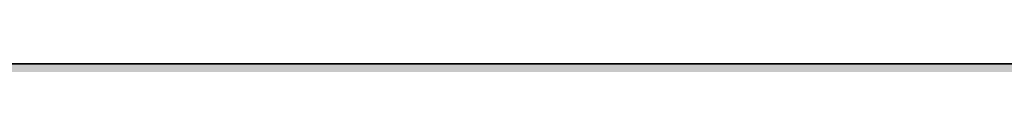
# Model space of a CAD drawing. Units: inches. Extents: x 2091 to 2899, y 967 to 2217.
# Tile 73 of 256: x 2214.757 to 2217.572, y 1099.919 to 1099.919. Entities that reach past the tile are written whole.
import ezdxf

# ---------------------------------------------------------------- set-up
doc = ezdxf.new("R2010")
doc.units = ezdxf.units.IN
doc.layers.add('A-WALL-PATT', color=141, linetype='Continuous', lineweight=13, true_color=0xadddf7)
doc.layers.add('L-SITE-WALL', color=7, linetype='Continuous', lineweight=35)

msp = doc.modelspace()

# ---------------------------------------------------------------- hatches: boundary and pattern name
at = {"layer": 'A-WALL-PATT'}
h = msp.add_hatch(color=256, dxfattribs=at)
h.dxf.hatch_style = 1
h.paths.add_polyline_path([(2212.1436, 1941.4191), (2387.6436, 1941.4191), (2387.6436, 1824.4191), (2392.1436, 1824.4191), (2392.1436, 1941.4191), (2609.6436, 1941.4191), (2609.6436, 1825.9191), (2614.1436, 1825.9191), (2614.1436, 1941.4191), (2794.1436, 1941.4191), (2794.1436, 1928.7622), (2803.1436, 1928.7622), (2803.1436, 2050.9191), (2203.1436, 2050.9191), (2203.1436, 1900.7579), (2212.1436, 1900.7579)])
h.paths.add_polyline_path([(2212.1436, 1945.9191), (2212.1436, 2041.9191), (2794.1436, 2041.9191), (2794.1436, 1945.9191), (2402.2482, 1945.9191), (2401.1024, 1945.7758), (2398.7024, 1945.7758)], flags=16)
h.paths.add_polyline_path([(2230.2299, 1948.0628), (2227.3499, 1949.5028), (2225.9099, 1951.9028), (2223.9899, 1952.8628), (2223.0299, 1955.2628), (2222.0699, 1959.5828), (2222.0699, 1963.4228), (2223.0299, 1965.6628), (2223.9899, 1965.3428), (2225.5859, 1963.8607), (2226.9115, 1964.9573), (2226.9489, 1965.9388), (2227.7783, 1966.9521), (2228.1999, 1968.8787), (2230.7099, 1964.8628), (2233.5899, 1966.3028), (2233.6073, 1966.3319), (2233.7727, 1964.9382), (2234.6338, 1963.6765), (2235.0299, 1963.9028), (2236.282, 1965.5724), (2235.9899, 1962.9428), (2237.9545, 1957.54), (2238.3899, 1957.9028), (2239.2159, 1960.3058), (2238.6546, 1966.385), (2238.6928, 1966.4381), (2238.8406, 1967.4997), (2238.7803, 1967.6875), (2238.8805, 1967.7868), (2238.6669, 1966.2518), (2239.2159, 1960.3058), (2238.3899, 1957.9028), (2236.9499, 1956.7028), (2234.5499, 1949.9828)], flags=0)
h.paths.add_polyline_path([(2278.012, 1948.0628), (2276.4964, 1947.8733), (2275.8498, 1947.6886), (2274.652, 1947.1028)], flags=0)
h.paths.add_polyline_path([(2269.852, 1955.7428), (2268.2762, 1956.6293), (2270.8673, 1956.3484), (2269.372, 1958.1428), (2268.715, 1959.1923), (2270.5698, 1958.7286), (2268.5807, 1961.9061), (2270.812, 1960.8919), (2270.812, 1963.4228), (2271.3933, 1964.7793), (2270.2918, 1966.1562), (2271.772, 1965.6628), (2272.1414, 1966.5248), (2273.9298, 1965.9286), (2275.6304, 1968.0543), (2276.3319, 1966.7219), (2276.5204, 1966.9521), (2276.942, 1968.8787), (2277.7343, 1967.6111), (2278.1399, 1969.4645), (2279.6591, 1967.0337), (2280.412, 1966.7828), (2280.9493, 1967.5888), (2281.6098, 1967.3686), (2282.1333, 1968.1538), (2282.3492, 1966.3334), (2282.3498, 1966.3326), (2283.4076, 1968.0954), (2283.7126, 1965.524), (2284.3202, 1964.6338), (2284.5118, 1964.8892), (2284.235, 1965.7048), (2284.5005, 1967.319), (2284.9079, 1965.4174), (2285.3963, 1966.0686), (2285.4328, 1966.2906), (2285.4733, 1966.1713), (2286.3539, 1967.3454), (2286.222, 1966.1582), (2287.6635, 1968.0802), (2287.714, 1968.4428), (2288.4816, 1969.0167), (2288.574, 1968.7289), (2288.9175, 1969.069), (2288.6068, 1966.8376), (2288.9287, 1963.3513), (2288.935, 1963.3568), (2288.9297, 1963.3404), (2289.0153, 1962.4139), (2290.1112, 1963.8751), (2290.1328, 1963.9426), (2290.2177, 1964.0171), (2290.1112, 1963.8751), (2289.1558, 1960.8916), (2288.594, 1959.2572), (2288.572, 1959.1028), (2289.532, 1960.5428), (2290.012, 1962.4628), (2290.1918, 1962.6427), (2289.7698, 1959.6886), (2286.8898, 1957.2886), (2284.4898, 1950.5686), (2283.3147, 1950.0463), (2283.292, 1949.9828), (2280.2901, 1948.6486), (2281.1298, 1948.6486), (2282.5698, 1948.1686), (2283.2047, 1948.0628), (2278.972, 1948.0628), (2276.092, 1949.5028), (2274.652, 1951.9028), (2272.732, 1952.8628)], flags=0)
h.paths.add_polyline_path([(2271.1589, 1958.0218), (2272.9698, 1955.8486), (2272.0098, 1960.1686), (2272.0098, 1964.0086), (2272.6244, 1965.4427), (2274.328, 1963.8607), (2275.6536, 1964.9573), (2275.6377, 1964.5391), (2277.4122, 1966.0069), (2277.033, 1965.1568), (2276.8299, 1964.9756), (2276.766, 1963.295), (2277.4496, 1962.6602), (2279.452, 1964.8628), (2282.332, 1966.3028), (2283.5298, 1966.8886), (2283.2945, 1966.7709), (2283.913, 1963.8847), (2284.8992, 1964.4483), (2284.732, 1962.9428), (2286.6966, 1957.54), (2287.132, 1957.9028), (2287.5419, 1959.0954), (2287.7794, 1958.4423), (2285.6827, 1956.6951), (2285.8765, 1959.7953), (2284.732, 1962.9428), (2284.8992, 1964.4483), (2283.913, 1963.8847), (2284.2238, 1962.4341), (2283.4244, 1963.6055), (2281.6098, 1962.5686), (2281.1298, 1960.1686), (2282.0898, 1956.3286), (2283.0498, 1952.9686), (2282.5698, 1950.5686), (2280.1698, 1948.6486), (2279.8833, 1948.7919), (2278.972, 1948.0628), (2278.972, 1949.0228), (2278.6723, 1949.3974), (2277.2898, 1950.0886), (2275.8498, 1952.4886), (2273.9298, 1953.4486), (2272.4898, 1954.8886), (2271.9216, 1954.8886), (2271.772, 1955.2628)], flags=0)
h.paths.add_polyline_path([(2311.9941, 1955.7428), (2312.0627, 1955.6742), (2312.0551, 1955.7085)], flags=0)
h.paths.add_polyline_path([(2331.9561, 1963.9518), (2333.3961, 1965.3918), (2331.0771, 1963.3568), (2330.9986, 1963.1115)], flags=0)
h.paths.add_polyline_path([(2310.5541, 1954.3028), (2307.0398, 1956.2799), (2310.7629, 1955.8763), (2312.4741, 1953.8228), (2313.4341, 1951.4228), (2315.3541, 1950.4628), (2316.7941, 1948.0628), (2317.4661, 1947.7268), (2319.3687, 1947.9646), (2317.7541, 1949.9828), (2317.5695, 1950.6105), (2316.7941, 1951.9028), (2314.8741, 1952.8628), (2313.9141, 1955.2628), (2311.5141, 1958.1428), (2309.3755, 1961.5592), (2311.5141, 1960.3371), (2311.5141, 1961.9828), (2310.6047, 1963.1196), (2311.7266, 1962.4785), (2312.4183, 1964.0926), (2312.256, 1964.2955), (2313.1941, 1963.9828), (2313.9141, 1965.6628), (2314.6468, 1965.4186), (2315.3541, 1966.3028), (2316.7941, 1967.7428), (2316.1574, 1966.9469), (2317.0341, 1965.2819), (2317.2226, 1965.5121), (2317.777, 1968.0458), (2318.4741, 1966.7219), (2318.6626, 1966.9521), (2319.0842, 1968.8787), (2321.207, 1965.4821), (2322.1614, 1966.9137), (2322.5541, 1966.7828), (2322.786, 1967.1306), (2322.8816, 1966.3243), (2323.312, 1965.7217), (2323.6513, 1965.8914), (2324.3965, 1967.1334), (2324.6569, 1964.9382), (2324.972, 1964.4766), (2325.3873, 1967.0015), (2325.9408, 1964.4183), (2327.2289, 1966.1358), (2327.1663, 1965.5724), (2328.0591, 1966.7628), (2328.2246, 1966.2475), (2329.668, 1967.6769), (2329.6646, 1967.6875), (2329.7648, 1967.7868), (2329.5511, 1966.2518), (2330.1001, 1960.3058), (2329.3328, 1958.0735), (2329.3131, 1957.9352), (2329.6341, 1958.2028), (2330.2341, 1959.1028), (2330.7141, 1961.0228), (2331.0341, 1961.3428), (2330.7141, 1959.1028), (2329.6341, 1958.2028), (2329.2741, 1957.6628), (2327.7121, 1956.3611), (2325.4341, 1949.9828), (2324.3338, 1949.4937), (2323.9941, 1948.5428), (2319.6741, 1946.6228), (2316.7941, 1948.0628), (2315.3541, 1950.4628), (2313.4341, 1951.4228)], flags=0)
h.paths.add_polyline_path([(2321.3357, 1947.952), (2321.1141, 1948.0628), (2321.1141, 1949.0228), (2319.1941, 1951.4228), (2316.7941, 1959.5828), (2316.6632, 1959.5828), (2315.3541, 1958.1428), (2314.3941, 1958.1428), (2313.1483, 1958.7091), (2312.9541, 1959.5828), (2312.9541, 1960.8919), (2315.8341, 1959.5828), (2316.6632, 1959.5828), (2317.3147, 1960.2994), (2315.0302, 1962.4207), (2316.3558, 1963.5173), (2316.3723, 1963.9516), (2316.4702, 1963.8607), (2317.7958, 1964.9573), (2317.7552, 1963.8897), (2319.1751, 1965.1568), (2319.4984, 1965.8814), (2321.1141, 1965.3428), (2323.2359, 1962.3724), (2325.6863, 1963.7726), (2325.5428, 1962.4806), (2325.1988, 1963.494), (2324.4785, 1963.0824), (2324.926, 1960.9941), (2324.0781, 1962.2365), (2322.4148, 1961.286), (2322.0741, 1959.5828), (2323.0341, 1955.7428), (2323.9941, 1952.3828), (2323.5141, 1949.9828), (2322.1427, 1948.8856), (2322.0741, 1948.5428)], flags=0)
h.paths.add_polyline_path([(2320.2075, 1963.3375), (2320.1541, 1963.4228), (2320.3941, 1963.5428)], flags=0)
h.paths.add_polyline_path([(2353.8505, 1965.8105), (2354.0305, 1965.7505), (2354.3305, 1966.4505), (2354.3305, 1966.9305)], flags=0)
h.paths.add_polyline_path([(2359.0206, 1969.0264), (2359.0984, 1968.9019), (2359.2335, 1969.5195), (2359.2335, 1969.9995)], flags=0)
h.paths.add_polyline_path([(2358.2567, 1966.6817), (2357.9836, 1966.348), (2358.2113, 1966.1462), (2358.4105, 1966.3896)], flags=0)
h.paths.add_polyline_path([(2357.7685, 1966.0588), (2357.7322, 1965.105), (2357.751, 1965.1206), (2357.7695, 1965.6065), (2357.7695, 1966.0578)], flags=0)
h.paths.add_polyline_path([(2359.1115, 1965.3045), (2359.1115, 1964.8245), (2359.8445, 1966.4675), (2359.8445, 1966.9475)], flags=0)
h.paths.add_polyline_path([(2360.2237, 1966.6214), (2360.6985, 1969.3625), (2360.6985, 1969.8425), (2360.2105, 1967.0255), (2360.2105, 1966.6425)], flags=0)
h.paths.add_polyline_path([(2363.4505, 1967.8905), (2363.4505, 1968.3705), (2362.4905, 1966.9305), (2362.656, 1966.6988)], flags=0)
h.paths.add_polyline_path([(2364.4755, 1966.0788), (2365.8505, 1968.3705), (2365.8505, 1968.8505), (2364.428, 1966.4796)], flags=0)
h.paths.add_polyline_path([(2366.3135, 1965.8525), (2366.3667, 1965.6958), (2366.8025, 1968.3455), (2366.8025, 1968.8255)], flags=0)
h.paths.add_polyline_path([(2367.1653, 1965.8035), (2367.2905, 1966.9305), (2367.2905, 1967.4105), (2367.1027, 1965.7201)], flags=0)
h.paths.add_polyline_path([(2370.0365, 1959.9735), (2371.0135, 1963.0245), (2371.0135, 1963.5045), (2370.0365, 1960.4535)], flags=0)
h.paths.add_polyline_path([(2371.6105, 1960.2105), (2372.5705, 1961.6505), (2372.5705, 1962.1305), (2371.8025, 1960.9785)], flags=0)
h.paths.add_polyline_path([(2350.8737, 1956.0051), (2351.9305, 1955.8905), (2354.4905, 1953.3305), (2353.8505, 1954.9305), (2351.4505, 1957.8105), (2347.9355, 1963.4255), (2347.9355, 1963.9055), (2351.4505, 1958.2905), (2353.7051, 1955.585), (2352.8905, 1959.2505), (2352.8905, 1959.7305), (2352.8905, 1961.9248), (2356.7305, 1959.7305), (2358.4545, 1961.6268), (2354.8105, 1965.0105), (2355.0309, 1965.2859), (2358.6911, 1961.8871), (2361.5305, 1965.0105), (2364.3765, 1966.4335), (2364.5244, 1965.1869), (2365.4545, 1963.8242), (2365.8811, 1964.068), (2365.3705, 1966.4505), (2365.3705, 1966.9305), (2366.8105, 1960.2105), (2366.8105, 1959.7305), (2366.3887, 1952.9814), (2367.7705, 1956.8505), (2368.6412, 1957.5761), (2366.8105, 1962.6105), (2366.8105, 1963.0905), (2368.7752, 1957.6877), (2369.2105, 1958.0505), (2370.0016, 1960.3519), (2369.4752, 1966.0527), (2369.5135, 1966.1058), (2369.5142, 1966.1109), (2369.4752, 1966.5327), (2369.5135, 1966.5858), (2369.6146, 1967.3126), (2369.1825, 1968.6585), (2369.1825, 1969.1385), (2369.601, 1967.8352), (2369.7012, 1967.9345), (2369.7179, 1968.0547), (2370.1452, 1968.3741), (2369.7787, 1968.0112), (2369.7012, 1967.4545), (2370.4682, 1968.214), (2369.6749, 1967.2658), (2369.5142, 1966.1109), (2370.0365, 1960.4535), (2370.0365, 1959.9735), (2369.4418, 1958.2432), (2370.6505, 1959.2505), (2371.0458, 1962.0176), (2371.1305, 1962.1305), (2370.6505, 1958.7705), (2367.7705, 1956.3705), (2365.3705, 1949.6505), (2362.0791, 1948.1876), (2363.4505, 1947.7305), (2361.0505, 1947.7305), (2360.0905, 1947.7305), (2357.1039, 1947.3572), (2360.0905, 1948.2105), (2358.1705, 1949.1705), (2356.7305, 1951.5705), (2354.8105, 1952.5305), (2351.9305, 1955.4105)], flags=0)
h.paths.add_polyline_path([(2361.0505, 1948.6905), (2359.1305, 1951.0905), (2356.7305, 1959.2505), (2355.7705, 1959.2505), (2352.8905, 1960.5596), (2352.8905, 1961.4448), (2355.8905, 1959.7305), (2356.7305, 1959.7305), (2356.8372, 1959.3678), (2361.5305, 1964.5305), (2363.2484, 1965.3894), (2364.9253, 1963.0418), (2362.4905, 1961.6505), (2362.0639, 1959.5172), (2362.9705, 1955.8905), (2363.9305, 1952.5305), (2363.9305, 1952.0505), (2363.4505, 1949.6505), (2361.0505, 1947.7305)], flags=0)
h.paths.add_polyline_path([(2359.1305, 1951.5705), (2359.2905, 1951.3705), (2361.0505, 1954.4505), (2361.0505, 1954.9305)], flags=0)
h.paths.add_polyline_path([(2357.2195, 1966.5455), (2356.7925, 1968.8145), (2356.7925, 1969.2945), (2357.2195, 1967.0255)], flags=0)
h.paths.add_polyline_path([(2361.0505, 1954.4505), (2361.5305, 1958.7705), (2361.5305, 1959.2505), (2361.0505, 1954.9305)], flags=0)
h.paths.add_polyline_path([(2402.5483, 1948.4861), (2402.3024, 1948.4158), (2402.5904, 1948.4158)], flags=0)
h.paths.add_polyline_path([(2394.1424, 1956.0958), (2395.6851, 1954.5532), (2396.7205, 1953.9707), (2396.0624, 1955.6158), (2395.2414, 1956.6011), (2395.8789, 1956.4417), (2395.1024, 1959.9358), (2395.1024, 1963.7758), (2396.0624, 1966.0158), (2397.0224, 1965.6958), (2398.6185, 1964.2138), (2399.9441, 1965.3103), (2399.9814, 1966.2918), (2400.8109, 1967.3052), (2401.2325, 1969.2317), (2403.5379, 1965.543), (2403.942, 1967.3893), (2404.7024, 1967.1358), (2405.4603, 1966.0748), (2406.6224, 1966.6558), (2406.6399, 1966.6849), (2406.8052, 1965.2912), (2406.9257, 1965.1147), (2407.3424, 1964.9758), (2407.8743, 1965.7737), (2408.1691, 1964.3981), (2409.3146, 1965.9254), (2409.2175, 1965.0511), (2409.4452, 1963.1312), (2410.3064, 1961.8695), (2410.7024, 1962.0958), (2411.4423, 1963.0823), (2411.1654, 1963.8978), (2411.6164, 1966.6398), (2411.7254, 1966.7911), (2411.8732, 1967.8527), (2411.8129, 1968.0405), (2411.9131, 1968.1398), (2411.6994, 1966.6048), (2412.2484, 1960.6588), (2413.2254, 1963.7098), (2414.3779, 1964.7212), (2414.5132, 1965.6927), (2414.4529, 1965.8805), (2414.5531, 1965.9798), (2414.3779, 1964.7212), (2414.5198, 1964.8457), (2414.3654, 1964.6311), (2414.3394, 1964.4448), (2414.8884, 1958.4988), (2414.0624, 1956.0958), (2412.6224, 1954.8958), (2410.1714, 1948.0329), (2410.0167, 1948.0844), (2405.9024, 1946.2558), (2405.9024, 1947.2158), (2405.2043, 1948.0886), (2404.2224, 1948.4158), (2403.2624, 1948.4158), (2400.3824, 1949.8558), (2399.6624, 1951.0558), (2397.9824, 1952.7358), (2397.0224, 1953.2158), (2395.6851, 1954.5532), (2392.6568, 1956.2569)], flags=0)
h.paths.add_polyline_path([(2409.0857, 1964.4074), (2409.1304, 1964.2757), (2409.2624, 1964.4958)], flags=0)
h.paths.add_polyline_path([(2397.7424, 1961.6158), (2398.7024, 1963.8558), (2399.6624, 1963.5358), (2401.4266, 1965.741), (2401.7914, 1966.5588), (2402.0714, 1965.0708), (2402.8355, 1964.3934), (2403.2624, 1964.9149), (2403.3381, 1964.7711), (2402.6155, 1963.9762), (2402.4986, 1960.9022), (2403.543, 1959.9325), (2404.4132, 1960.8897), (2404.7024, 1962.3358), (2407.9163, 1964.1724), (2409.5202, 1961.9269), (2410.9871, 1957.893), (2411.4224, 1958.2558), (2412.048, 1960.0756), (2412.4103, 1959.0791), (2411.6756, 1958.4668), (2411.6624, 1958.2558), (2411.6261, 1958.4255), (2409.9824, 1957.0558), (2407.5824, 1950.3358), (2403.2624, 1948.4158), (2403.2624, 1949.3758), (2401.3424, 1951.7758), (2399.4165, 1958.324), (2397.7424, 1959.0849), (2397.7424, 1959.9701), (2397.1024, 1960.3358), (2397.7424, 1960.0449)], flags=0)
h.paths.add_polyline_path([(2405.9024, 1952.9758), (2405.9504, 1953.4078), (2406.0167, 1953.1758)], flags=0)
h.paths.add_polyline_path([(2449.8178, 1967.114), (2449.7523, 1967.1358), (2449.7937, 1967.0779)], flags=0)
h.paths.add_polyline_path([(2451.6977, 1966.6181), (2451.7409, 1966.6901), (2451.6921, 1966.6657)], flags=0)
h.paths.add_polyline_path([(2454.3436, 1965.7376), (2455.7523, 1967.6158), (2455.9923, 1968.0958), (2454.3645, 1965.9254)], flags=0)
h.paths.add_polyline_path([(2457.5473, 1968.8638), (2457.7873, 1969.3438), (2457.0543, 1968.7958), (2457.0076, 1968.4603)], flags=0)
h.paths.add_polyline_path([(2456.9218, 1967.8567), (2456.8022, 1968.229), (2456.723, 1967.6598)], flags=0)
h.paths.add_polyline_path([(2457.3023, 1967.3768), (2457.5423, 1967.8568), (2456.8103, 1966.8398), (2456.7405, 1966.7002), (2456.749, 1966.6081)], flags=0)
h.paths.add_polyline_path([(2458.2753, 1963.7098), (2458.1553, 1963.3352), (2460.3543, 1965.2648), (2460.5943, 1965.7448)], flags=0)
h.paths.add_polyline_path([(2458.3923, 1962.8158), (2458.3641, 1962.6182), (2459.5923, 1964.2558), (2459.8323, 1964.7358)], flags=0)
h.paths.add_polyline_path([(2459.3523, 1962.8158), (2459.2723, 1962.4958), (2460.0723, 1963.2958), (2460.3123, 1963.7758)], flags=0)
h.paths.add_polyline_path([(2458.6803, 1960.6078), (2458.6323, 1960.4158), (2459.5923, 1961.8558), (2459.8323, 1962.3358)], flags=0)
h.paths.add_polyline_path([(2437.8382, 1956.2427), (2439.1923, 1956.0958), (2441.3523, 1953.9358), (2440.8723, 1955.1358), (2438.4723, 1958.0158), (2438.0716, 1958.656), (2438.7123, 1958.4958), (2440.6396, 1956.1831), (2439.9123, 1959.4558), (2439.9123, 1963.2958), (2441.3523, 1966.6558), (2441.5923, 1967.1358), (2441.1123, 1966.0158), (2442.0723, 1965.6958), (2443.989, 1968.0917), (2444.2413, 1966.7508), (2444.9168, 1966.1519), (2445.6766, 1967.0801), (2446.2553, 1969.7248), (2446.4953, 1970.2048), (2446.2824, 1969.2317), (2447.3627, 1967.5033), (2447.7203, 1969.5678), (2447.9603, 1970.0478), (2447.4855, 1967.3068), (2448.7923, 1965.2158), (2448.4723, 1964.8638), (2448.5523, 1964.7358), (2451.4521, 1966.1857), (2451.6151, 1964.8112), (2452.3079, 1963.7962), (2453.2345, 1964.3257), (2454.0723, 1960.4158), (2453.6287, 1953.3177), (2454.7923, 1956.5758), (2455.0323, 1957.0558), (2455.7188, 1957.6279), (2453.8323, 1962.8158), (2453.941, 1963.7936), (2453.3353, 1965.5778), (2453.8243, 1968.5508), (2454.0643, 1969.0308), (2453.5753, 1966.0578), (2454.0403, 1964.6879), (2453.8323, 1962.8158), (2455.7188, 1957.6279), (2456.3672, 1958.1682), (2457.0583, 1960.1788), (2457.2983, 1960.6588), (2456.4723, 1958.2558), (2457.7177, 1959.2937), (2457.6723, 1958.9758), (2454.89, 1956.6572), (2453.6141, 1953.0849), (2453.5923, 1952.7358), (2453.3523, 1952.2558), (2453.3596, 1952.3722), (2452.6323, 1950.3358), (2452.3923, 1949.8558), (2449.2038, 1948.4387), (2450.7123, 1947.9358), (2448.0723, 1947.9358), (2447.1123, 1947.9358), (2444.5523, 1947.6158), (2447.1996, 1948.3722), (2445.1923, 1949.3758), (2443.7523, 1951.7758), (2441.8323, 1952.7358), (2438.9523, 1955.6158)], flags=0)
h.paths.add_polyline_path([(2443.9923, 1959.9358), (2444.0403, 1959.7726), (2444.1216, 1959.862)], flags=0)
h.paths.add_polyline_path([(2442.9123, 1959.9358), (2443.0323, 1959.9358), (2442.4457, 1960.2025)], flags=0)
h.paths.add_polyline_path([(2444.9829, 1965.0197), (2445.2793, 1965.2648), (2445.5193, 1965.7448), (2444.994, 1965.3103)], flags=0)
h.paths.add_polyline_path([(2446.1333, 1965.0298), (2446.3304, 1965.4715), (2444.9703, 1964.2578), (2444.7303, 1963.7778)], flags=0)
h.paths.add_polyline_path([(2442.7923, 1959.4558), (2443.7523, 1959.4558), (2446.1523, 1951.2958), (2446.4123, 1951.7508), (2446.3923, 1951.7758), (2448.0806, 1954.7303), (2448.5523, 1958.9758), (2441.8323, 1965.2158), (2442.1549, 1965.6191), (2448.7923, 1959.4558), (2448.3123, 1955.1358), (2448.0723, 1954.6558), (2446.4123, 1951.7508), (2448.3123, 1949.3758), (2448.3123, 1948.4158), (2450.5409, 1950.1987), (2450.9523, 1952.2558), (2449.9923, 1955.6158), (2449.0323, 1959.4558), (2449.5123, 1961.8558), (2449.7523, 1962.3358), (2449.6749, 1961.9487), (2452.9945, 1963.8457), (2453.0644, 1963.5194), (2452.8846, 1963.7829), (2449.6749, 1961.9487), (2449.2723, 1959.9358), (2450.2323, 1956.0958), (2451.1923, 1952.7358), (2450.7123, 1950.3358), (2450.4723, 1949.8558), (2448.0723, 1947.9358), (2448.0723, 1948.5358), (2445.4323, 1949.8558), (2443.9923, 1952.2558), (2442.0723, 1953.2158), (2441.1123, 1955.6158), (2440.1523, 1959.9358), (2440.1523, 1960.6558)], flags=0)
h.paths.add_polyline_path([(2456.6923, 1966.9858), (2457.6083, 1968.0808), (2457.8483, 1968.5608), (2456.9323, 1967.4658)], flags=0)
h.paths.add_polyline_path([(2489.8966, 1966.5802), (2489.9429, 1966.1893), (2490.7475, 1967.5302), (2491.3191, 1968.9512)], flags=0)
h.paths.add_polyline_path([(2473.5625, 1956.4071), (2477.14, 1956.0193), (2476.9553, 1956.2408), (2475.108, 1957.2801), (2476.3475, 1956.9702), (2475.1869, 1958.8242), (2476.9191, 1958.3912), (2475.4116, 1960.7993), (2477.7875, 1959.7193), (2477.7875, 1962.2502), (2477.6374, 1962.4379), (2477.8226, 1962.3321), (2478.3591, 1963.5841), (2478.3591, 1963.6712), (2477.3243, 1964.9646), (2478.7148, 1964.5011), (2479.3191, 1965.9112), (2480.2791, 1965.5912), (2481.784, 1967.4722), (2482.1165, 1965.7052), (2482.8806, 1965.0278), (2483.2093, 1965.4294), (2483.2202, 1965.7151), (2483.0759, 1965.989), (2483.7118, 1966.7658), (2484.1305, 1968.6792), (2484.7021, 1970.1002), (2484.4892, 1969.1271), (2486.5029, 1965.9051), (2487.3875, 1965.6102), (2488.1534, 1966.7591), (2488.717, 1965.9701), (2489.2001, 1966.2116), (2489.3307, 1965.111), (2490.3939, 1963.6225), (2490.6608, 1963.775), (2490.4939, 1964.5536), (2490.9231, 1963.9248), (2491.3191, 1964.1512), (2491.3334, 1964.1702), (2491.2105, 1964.5322), (2491.2818, 1964.9655), (2491.4258, 1964.2934), (2494.0765, 1967.8276), (2494.4979, 1966.5149), (2494.5982, 1966.6142), (2494.6895, 1967.2702), (2495.1067, 1967.5822), (2495.1298, 1967.7481), (2495.0696, 1967.9359), (2495.1698, 1968.0351), (2495.0318, 1967.0436), (2495.7538, 1967.7587), (2494.9821, 1966.6864), (2494.9561, 1966.5002), (2495.479, 1960.8369), (2495.9105, 1962.1842), (2496.4821, 1963.6052), (2496.0727, 1962.3266), (2496.7689, 1962.9375), (2496.5991, 1962.7112), (2496.1191, 1959.3512), (2496.7329, 1960.2718), (2496.9875, 1961.2902), (2497.5591, 1962.7112), (2497.0791, 1960.7912), (2496.5075, 1959.3702), (2495.5475, 1957.9302), (2492.7588, 1955.6064), (2490.8391, 1950.2312), (2490.2675, 1948.8102), (2485.9475, 1946.8902), (2483.0675, 1948.3302), (2481.6275, 1950.7302), (2479.7075, 1951.6902), (2476.8275, 1954.5702)], flags=0)
h.paths.add_polyline_path([(2485.577, 1948.3134), (2485.5591, 1948.3112), (2485.5788, 1948.3112)], flags=0)
h.paths.add_polyline_path([(2478.6451, 1954.5512), (2478.109, 1956.9633), (2479.3191, 1955.5112), (2480.2791, 1953.1112), (2482.1991, 1952.1512), (2483.6391, 1949.7512), (2486.5191, 1948.3112), (2486.5191, 1949.2712), (2484.7393, 1951.4959), (2484.0275, 1950.2502), (2481.6275, 1958.4102), (2482.3751, 1959.2327), (2482.1991, 1959.8312), (2483.1976, 1960.9295), (2479.7075, 1964.1702), (2480.6034, 1965.2901), (2481.8752, 1964.1091), (2482.6664, 1964.7636), (2482.6154, 1963.4218), (2482.9892, 1963.0747), (2484.0085, 1963.9842), (2484.6836, 1965.4975), (2484.5801, 1965.4052), (2485.3573, 1967.1471), (2485.1206, 1965.7812), (2486.4275, 1963.6902), (2488.1454, 1964.5492), (2489.8223, 1962.2016), (2490.7475, 1962.7302), (2491.9997, 1964.3998), (2492.076, 1965.0873), (2492.2129, 1964.6841), (2492.4854, 1965.0474), (2492.2791, 1963.1912), (2494.2438, 1957.7884), (2494.5625, 1958.054), (2494.9335, 1959.1332), (2495.5051, 1960.5542), (2494.6791, 1958.1512), (2494.1075, 1956.7302), (2494.5625, 1958.054), (2493.4085, 1957.0923), (2491.7075, 1961.7702), (2491.9997, 1964.3998), (2490.7475, 1962.7302), (2487.712, 1960.9957), (2487.4791, 1959.8312), (2488.4391, 1955.9912), (2489.3991, 1952.6312), (2488.9191, 1950.2312), (2488.5769, 1949.9574), (2488.3475, 1948.8102), (2487.6517, 1948.2536), (2487.4791, 1948.3112), (2486.5191, 1948.3112), (2483.6391, 1949.7512), (2482.1991, 1952.1512), (2480.2791, 1953.1112), (2478.8391, 1954.5512)], flags=0)
h.paths.add_polyline_path([(2526.6483, 1966.9875), (2526.5173, 1967.0312), (2526.6001, 1966.9153)], flags=0)
h.paths.add_polyline_path([(2528.4706, 1966.4467), (2528.5745, 1966.6197), (2528.4571, 1966.561)], flags=0)
h.paths.add_polyline_path([(2534.1333, 1967.4962), (2534.1567, 1967.5428), (2534.0598, 1967.4083)], flags=0)
h.paths.add_polyline_path([(2536.1619, 1964.0506), (2535.1573, 1962.7112), (2535.1009, 1962.3159), (2536.1173, 1963.6712), (2536.4205, 1964.2775)], flags=0)
h.paths.add_polyline_path([(2535.1573, 1959.8312), (2536.1173, 1961.2712), (2536.5973, 1962.2312), (2535.2533, 1960.2152)], flags=0)
h.paths.add_polyline_path([(2513.249, 1956.2848), (2516.2212, 1955.9626), (2514.9973, 1957.4312), (2514.1958, 1958.7115), (2515.4773, 1958.3912), (2516.9319, 1956.6457), (2516.4373, 1958.8712), (2516.4373, 1962.7112), (2516.8727, 1963.727), (2515.3464, 1965.6348), (2517.3973, 1964.9512), (2517.8773, 1966.0712), (2518.3573, 1967.0312), (2517.8773, 1965.9112), (2518.8373, 1965.5912), (2520.4866, 1967.6527), (2520.7663, 1966.1662), (2521.5304, 1965.4887), (2521.7814, 1965.7954), (2521.8009, 1966.3073), (2521.4778, 1966.9209), (2521.2463, 1967.1262), (2521.1777, 1967.4909), (2521.4778, 1966.9209), (2522.0104, 1966.4487), (2522.2574, 1966.7504), (2522.7803, 1969.1402), (2523.2603, 1970.1002), (2523.0474, 1969.1271), (2524.6731, 1966.5259), (2526.0373, 1966.0712), (2526.7952, 1965.0101), (2527.9771, 1965.601), (2528.1401, 1964.2266), (2528.6646, 1963.4582), (2529.3886, 1963.8719), (2529.3297, 1964.147), (2529.4813, 1963.9248), (2529.8773, 1964.1512), (2529.984, 1964.2934), (2529.7891, 1965.2032), (2530.0624, 1964.3979), (2532.8025, 1968.0513), (2533.1478, 1966.9759), (2533.248, 1967.0751), (2533.3393, 1967.7312), (2533.6728, 1967.9805), (2533.728, 1968.0351), (2533.5143, 1966.5002), (2534.0247, 1960.9725), (2534.5603, 1962.6452), (2535.0403, 1963.6052), (2534.0633, 1960.5542), (2533.2373, 1958.1512), (2534.2882, 1959.0268), (2534.1973, 1958.3912), (2531.5126, 1956.1539), (2529.3973, 1950.2312), (2528.9173, 1949.2712), (2526.4488, 1948.174), (2527.4773, 1947.8312), (2530.3573, 1947.3512), (2524.5973, 1947.3512), (2521.7173, 1948.7912), (2520.2773, 1951.1912), (2518.3573, 1952.1512), (2515.4773, 1955.0312)], flags=0)
h.paths.add_polyline_path([(2523.9348, 1967.1903), (2523.6195, 1966.4837), (2523.7705, 1966.2421)], flags=0)
h.paths.add_polyline_path([(2518.8373, 1953.1112), (2517.8773, 1955.5112), (2516.885, 1959.9768), (2516.9173, 1959.9621), (2516.9173, 1962.0254), (2520.7573, 1959.8312), (2522.0249, 1961.2255), (2518.3573, 1964.6312), (2519.0026, 1965.4377), (2520.4334, 1964.1091), (2521.3011, 1964.8269), (2521.2452, 1963.3553), (2525.6383, 1959.276), (2526.0373, 1961.2712), (2529.3973, 1963.1912), (2530.6495, 1964.8607), (2530.6647, 1964.9976), (2530.692, 1964.9173), (2531.0878, 1965.4451), (2530.946, 1964.1689), (2530.692, 1964.9173), (2529.3973, 1963.1912), (2526.3625, 1961.457), (2526.0373, 1959.8312), (2526.9973, 1955.9912), (2527.9573, 1952.6312), (2527.4773, 1950.2312), (2527.1345, 1949.9569), (2526.9739, 1949.1541), (2526.6973, 1949.0312), (2524.5973, 1947.3512), (2524.5973, 1948.3112), (2524.2773, 1948.7112), (2522.1973, 1949.7512), (2520.7573, 1952.1512)], flags=0)
h.paths.add_polyline_path([(2520.2773, 1958.8712), (2520.8533, 1959.5048), (2523.1573, 1951.6712), (2524.6139, 1954.2201), (2524.5973, 1954.0712), (2522.6773, 1950.7112)], flags=0)
h.paths.add_polyline_path([(2559.3709, 1966.3112), (2559.3984, 1966.3249), (2559.4019, 1966.3453)], flags=0)
h.paths.add_polyline_path([(2549.7709, 1957.1912), (2552.6509, 1954.3112), (2552.134, 1955.6035), (2550.6109, 1957.4312), (2547.0959, 1963.0462), (2545.7759, 1965.2062), (2549.2909, 1959.5912), (2551.6909, 1956.7112), (2550.7929, 1960.7521), (2550.7309, 1960.7803), (2550.7309, 1964.8712), (2551.6909, 1967.1112), (2552.6509, 1966.7912), (2554.247, 1965.3091), (2555.0343, 1965.9603), (2555.5817, 1966.6446), (2555.6099, 1967.3872), (2556.4394, 1968.4005), (2556.861, 1970.3271), (2559.3709, 1966.3112), (2560.6909, 1964.1512), (2562.4088, 1965.0101), (2561.6509, 1966.0712), (2560.3309, 1968.2312), (2561.7585, 1966.2325), (2562.3472, 1967.1156), (2562.4337, 1966.3866), (2563.1278, 1965.3696), (2563.5709, 1965.5912), (2563.5884, 1965.6202), (2563.3625, 1967.5235), (2563.7225, 1965.8438), (2565.06, 1968.073), (2564.7329, 1965.1287), (2565.1176, 1963.3334), (2567.4446, 1966.4361), (2567.3156, 1967.8333), (2567.3538, 1967.8864), (2567.5016, 1968.9481), (2567.4413, 1969.1359), (2567.5416, 1969.2351), (2567.3279, 1967.7002), (2567.8769, 1961.7542), (2568.7467, 1964.4703), (2568.6356, 1965.6733), (2568.6738, 1965.7264), (2568.8216, 1966.7881), (2568.7613, 1966.9759), (2568.8616, 1967.0751), (2568.6479, 1965.5402), (2568.7261, 1964.693), (2568.8539, 1964.8052), (2568.7467, 1964.4703), (2568.8172, 1963.7063), (2568.9709, 1963.9112), (2568.8661, 1963.1773), (2569.1969, 1959.5942), (2568.3709, 1957.1912), (2566.9309, 1955.9912), (2564.6203, 1949.5214), (2564.6509, 1949.5112), (2564.6166, 1949.5112), (2564.5309, 1949.2712), (2560.2109, 1947.3512), (2557.3309, 1948.7912), (2556.0452, 1950.934), (2556.0109, 1950.9512), (2555.8566, 1951.2083), (2553.9709, 1952.1512), (2551.0909, 1955.0312), (2546.6501, 1957.5295)], flags=0)
h.paths.add_polyline_path([(2567.0258, 1959.3302), (2567.035, 1959.3049), (2567.0509, 1959.3512)], flags=0)
h.paths.add_polyline_path([(2551.9683, 1962.5184), (2553.0109, 1964.9512), (2553.9709, 1964.6312), (2555.567, 1963.1491), (2556.8926, 1964.2456), (2556.9299, 1965.2272), (2557.144, 1965.4887), (2556.4201, 1966.1306), (2556.3914, 1966.105), (2556.3799, 1966.1662), (2556.4201, 1966.1306), (2556.9519, 1966.6052), (2557.0921, 1966.9195), (2557.5709, 1966.0102), (2557.7594, 1966.2405), (2557.4179, 1964.6802), (2556.8926, 1964.2456), (2556.8071, 1961.9976), (2560.6909, 1958.3912), (2560.6355, 1957.8927), (2560.8109, 1957.1912), (2561.7709, 1953.8312), (2561.2909, 1951.4312), (2559.1104, 1949.6868), (2559.1565, 1949.6292), (2563.0265, 1951.3492), (2562.6109, 1949.2712), (2560.2109, 1947.3512), (2560.2109, 1948.3112), (2559.2509, 1949.5112), (2558.8909, 1949.5112), (2558.8909, 1949.9612), (2558.2909, 1950.7112), (2558.0537, 1951.5177), (2556.9709, 1952.8712), (2555.0679, 1959.3415), (2552.0509, 1961.0654), (2552.0509, 1962.4712)], flags=0)
h.paths.add_polyline_path([(2588.33, 1958.3912), (2588.6102, 1958.111), (2588.5534, 1958.3669)], flags=0)
h.paths.add_polyline_path([(2594.7455, 1950.4931), (2593.9575, 1953.172), (2593.13, 1954.5512), (2591.21, 1955.5112), (2590.25, 1957.9112), (2588.309, 1960.2404), (2586.1773, 1961.2093), (2587.85, 1960.7912), (2587.2534, 1961.7442), (2588.4413, 1961.0654), (2588.4413, 1962.6555), (2588.4217, 1962.6653), (2588.4413, 1962.7112), (2586.914, 1964.6203), (2588.8771, 1963.728), (2589.29, 1964.6915), (2589.29, 1966.0712), (2590.25, 1968.3112), (2591.21, 1967.9912), (2592.8061, 1966.5091), (2594.1317, 1967.6056), (2594.169, 1968.5872), (2594.9985, 1969.6005), (2595.4201, 1971.5271), (2597.93, 1967.5112), (2600.81, 1968.9512), (2600.8275, 1968.9802), (2600.9928, 1967.5866), (2601.854, 1966.3248), (2602.1071, 1966.4695), (2602.2364, 1967.2551), (2602.3567, 1966.6934), (2603.5022, 1968.2207), (2603.21, 1965.5912), (2605.1747, 1960.1884), (2605.5069, 1960.4652), (2605.026, 1965.6733), (2605.0642, 1965.7264), (2605.212, 1966.7881), (2605.1517, 1966.9759), (2605.252, 1967.0751), (2605.3433, 1967.7312), (2605.9529, 1968.1869), (2605.8748, 1969.0333), (2605.913, 1969.0864), (2606.0608, 1970.1481), (2606.0005, 1970.3359), (2606.1007, 1970.4351), (2605.887, 1968.9002), (2606.436, 1962.9542), (2605.61, 1960.5512), (2605.997, 1960.8737), (2606.5643, 1962.6452), (2608.2415, 1964.1169), (2608.01, 1963.1912), (2607.05, 1961.7512), (2606.6315, 1961.4024), (2606.2013, 1958.3912), (2603.3213, 1955.9912), (2600.9213, 1949.2712), (2596.6013, 1947.3512), (2593.7213, 1948.7912), (2592.8573, 1950.2312), (2592.65, 1950.2312)], flags=0)
h.paths.add_polyline_path([(2596.6013, 1947.3512), (2596.6013, 1948.3112), (2594.6813, 1950.7112), (2596.155, 1953.29), (2595.53, 1954.0712), (2593.1992, 1961.996), (2592.6513, 1962.5047), (2591.7802, 1963.0025), (2593.283, 1964.2456), (2593.3203, 1965.2272), (2594.1498, 1966.2405), (2594.5714, 1968.1671), (2596.1827, 1965.589), (2596.9513, 1966.4345), (2598.0413, 1966.0712), (2598.7992, 1965.0101), (2599.9613, 1965.5912), (2599.9788, 1965.6202), (2600.1441, 1964.2266), (2601.0053, 1962.9648), (2601.4013, 1963.1912), (2602.6535, 1964.8607), (2602.3613, 1962.2312), (2603.7927, 1958.2947), (2601.9776, 1953.2124), (2601.9462, 1952.7095), (2599.4688, 1951.6084), (2599.0013, 1949.2712)], flags=0)
h.paths.add_polyline_path([(2597.5613, 1958.8712), (2597.671, 1959.4194), (2597.5951, 1958.7362)], flags=0)
h.paths.add_polyline_path([(2623.6663, 1961.2544), (2625.5192, 1960.7912), (2624.9655, 1961.6755), (2627.1992, 1960.6603), (2627.1992, 1961.1512), (2626.9592, 1962.2312), (2626.9592, 1963.4912), (2625.5823, 1965.2122), (2626.9592, 1964.4254), (2626.9592, 1965.8312), (2626.8692, 1965.8612), (2627.9192, 1968.3112), (2628.8792, 1967.9912), (2630.4752, 1966.5091), (2631.8008, 1967.6056), (2631.8382, 1968.5872), (2632.6676, 1969.6005), (2633.0892, 1971.5271), (2635.5992, 1967.5112), (2638.4792, 1968.9512), (2638.4966, 1968.9802), (2638.662, 1967.5866), (2639.1763, 1966.833), (2639.7802, 1967.8396), (2640.0258, 1966.6934), (2641.1713, 1968.2207), (2640.8792, 1965.5912), (2641.1143, 1964.9446), (2641.4113, 1965.3407), (2641.3081, 1964.4116), (2642.8438, 1960.1884), (2643.2792, 1960.5512), (2644.0847, 1962.8947), (2643.7839, 1966.1533), (2643.8068, 1966.1852), (2643.6007, 1968.4181), (2643.5228, 1968.6606), (2643.7299, 1970.1481), (2643.6696, 1970.3359), (2643.7698, 1970.4351), (2643.5562, 1968.9002), (2643.6007, 1968.4181), (2643.9096, 1967.4559), (2644.0098, 1967.5551), (2643.8117, 1966.1321), (2644.1052, 1962.9542), (2644.2388, 1961.3508), (2644.7192, 1961.7512), (2645.0329, 1962.2217), (2645.3222, 1963.1252), (2646.0764, 1963.787), (2645.0329, 1962.2217), (2644.3452, 1960.0742), (2643.5192, 1957.6712), (2642.0792, 1956.4712), (2639.7196, 1949.8644), (2639.8755, 1949.8384), (2635.3592, 1947.8312), (2632.4792, 1949.2712), (2631.0392, 1951.6712), (2629.1192, 1952.6312), (2628.1592, 1955.0312), (2625.7592, 1957.9112)], flags=0)
h.paths.add_polyline_path([(2627.8163, 1956.574), (2627.3737, 1958.5657), (2626.3763, 1959.7626), (2627.1992, 1959.3512), (2627.3737, 1958.5657), (2627.9192, 1957.9112), (2628.8792, 1955.5112), (2630.7992, 1954.5512), (2632.2392, 1952.1512), (2633.315, 1951.6132), (2631.0392, 1959.3512), (2631.4978, 1959.8557), (2630.7992, 1962.2312), (2631.4499, 1962.9469), (2630.7152, 1963.6291), (2632.0408, 1964.7256), (2632.0782, 1965.7072), (2632.2922, 1965.9687), (2631.7053, 1966.4891), (2633.1364, 1967.7661), (2633.3292, 1968.6471), (2634.6747, 1966.4943), (2635.2085, 1967.0814), (2636.7992, 1966.5512), (2637.6764, 1967.867), (2638.9939, 1966.0225), (2639.7053, 1966.429), (2641.1192, 1959.8312), (2640.9301, 1956.8057), (2639.4392, 1952.6312), (2638.2275, 1952.0926), (2637.7592, 1949.7512), (2635.3592, 1947.8312), (2635.3592, 1948.7912), (2633.4392, 1951.1912), (2633.315, 1951.6132), (2632.2392, 1952.1512), (2630.7992, 1954.5512), (2628.8792, 1955.5112)], flags=0)
h.paths.add_polyline_path([(2637.7592, 1953.8312), (2637.2792, 1955.5112), (2636.3192, 1959.3512), (2636.7992, 1961.7512), (2639.2339, 1963.1425), (2637.5571, 1965.4901), (2638.7389, 1966.081), (2638.902, 1964.7066), (2639.7631, 1963.4448), (2636.7992, 1961.7512), (2636.5325, 1960.4178), (2637.0392, 1958.3912), (2637.9992, 1955.0312)], flags=0)
h.paths.add_polyline_path([(2668.5674, 1951.4312), (2667.6074, 1953.8312), (2665.2074, 1956.7112), (2662.2939, 1961.3653), (2665.4474, 1959.5912), (2666.6474, 1958.3912), (2666.6474, 1959.9752), (2666.0583, 1960.6821), (2666.6474, 1960.3454), (2666.6474, 1961.9912), (2666.7001, 1962.1141), (2666.4074, 1963.4312), (2666.4074, 1967.2712), (2667.3674, 1969.5112), (2668.3274, 1969.1912), (2669.9235, 1967.7091), (2671.2491, 1968.8056), (2671.2864, 1969.7872), (2672.1159, 1970.8005), (2672.5375, 1972.7271), (2675.0474, 1968.7112), (2677.9274, 1970.1512), (2677.9449, 1970.1802), (2678.1102, 1968.7866), (2678.9713, 1967.5248), (2679.3674, 1967.7512), (2680.6196, 1969.4207), (2680.3274, 1966.7912), (2682.2921, 1961.3884), (2682.7274, 1961.7512), (2683.3583, 1963.5866), (2683.2321, 1964.9533), (2683.2703, 1965.0064), (2683.3932, 1965.8891), (2683.36, 1966.2492), (2683.3578, 1966.2559), (2683.3592, 1966.2572), (2682.9921, 1970.2333), (2683.0303, 1970.2864), (2683.1781, 1971.3481), (2683.1178, 1971.5359), (2683.2181, 1971.6351), (2683.0044, 1970.1002), (2683.3592, 1966.2572), (2683.4581, 1966.3551), (2683.3932, 1965.8891), (2683.4139, 1965.665), (2684.4238, 1966.8723), (2683.5534, 1964.1542), (2683.3583, 1963.5866), (2683.7934, 1958.8742), (2682.9674, 1956.4712), (2681.5274, 1955.2712), (2680.1092, 1951.3003), (2680.0849, 1950.9116), (2679.9768, 1950.9296), (2679.1274, 1948.5512), (2674.8074, 1946.6312), (2671.9274, 1948.0712), (2670.4874, 1950.4712)], flags=0)
h.paths.add_polyline_path([(2671.9357, 1953.227), (2671.6874, 1953.3512), (2670.2474, 1955.7512), (2668.3274, 1956.7112), (2667.3567, 1959.1378), (2669.5274, 1958.1512), (2670.4874, 1958.1512), (2671.4794, 1959.2424), (2670.6844, 1961.9454), (2668.8896, 1963.612), (2667.3074, 1964.3312), (2668.5674, 1963.9112), (2668.8309, 1964.2406), (2670.2474, 1963.4312), (2672.4221, 1965.8234), (2672.7775, 1967.4471), (2673.2341, 1966.7165), (2674.4119, 1968.0121), (2673.9806, 1965.5221), (2675.2874, 1963.4312), (2675.5541, 1963.5645), (2675.9324, 1965.4562), (2676.2474, 1965.3512), (2677.0053, 1964.2901), (2678.1674, 1964.8712), (2679.6074, 1967.2712), (2680.3274, 1963.9112), (2680.3066, 1963.5775), (2680.3472, 1963.4576), (2680.8596, 1964.1407), (2680.5674, 1961.5112), (2681.1036, 1960.0366), (2678.8874, 1953.8312), (2677.0925, 1953.0334), (2677.6874, 1950.9512), (2677.2074, 1948.5512), (2674.8074, 1946.6312), (2674.8074, 1947.5912), (2672.8874, 1949.9912)], flags=0)
h.paths.add_polyline_path([(2673.9846, 1951.9112), (2674.5674, 1952.9312), (2674.5674, 1951.9112), (2676.9674, 1953.8312), (2677.4474, 1956.2312), (2676.4874, 1959.5912), (2676.2474, 1960.5512), (2679.7296, 1962.541), (2680.0593, 1961.0025), (2679.2113, 1962.2448), (2676.2474, 1960.5512), (2676.4874, 1959.5912), (2677.4474, 1956.2312), (2676.9674, 1953.8312), (2674.5674, 1951.9112)], flags=0)
h.paths.add_polyline_path([(2707.4793, 1952.8147), (2706.5193, 1955.2147), (2705.5593, 1959.5347), (2705.5593, 1963.3747), (2706.5193, 1965.6147), (2707.4793, 1965.2947), (2709.0753, 1963.8126), (2710.401, 1964.9091), (2710.4383, 1965.8907), (2711.2677, 1966.904), (2711.6893, 1968.8306), (2714.1993, 1964.8147), (2717.0793, 1966.2547), (2717.0967, 1966.2837), (2717.2621, 1964.8901), (2718.1232, 1963.6283), (2718.5193, 1963.8547), (2719.7715, 1965.5242), (2719.4793, 1962.8947), (2721.4439, 1957.4919), (2721.8793, 1957.8547), (2722.7053, 1960.2577), (2722.144, 1966.3368), (2722.1822, 1966.3899), (2722.33, 1967.4516), (2722.2697, 1967.6393), (2722.37, 1967.7386), (2722.1563, 1966.2037), (2722.7053, 1960.2577), (2721.8793, 1957.8547), (2720.4393, 1956.6547), (2718.0393, 1949.9347), (2713.7193, 1948.0147), (2710.8393, 1949.4547), (2709.3993, 1951.8547)], flags=0)
h.paths.add_polyline_path([(2749.3012, 1952.8147), (2748.3412, 1955.2147), (2747.3812, 1959.5347), (2747.3812, 1963.3747), (2748.3412, 1965.6147), (2749.3012, 1965.2947), (2750.8973, 1963.8126), (2752.2229, 1964.9091), (2752.2602, 1965.8907), (2753.0897, 1966.904), (2753.5113, 1968.8306), (2756.0212, 1964.8147), (2758.9012, 1966.2547), (2758.9187, 1966.2837), (2759.084, 1964.8901), (2759.9452, 1963.6283), (2760.3412, 1963.8547), (2761.5934, 1965.5242), (2761.3012, 1962.8947), (2763.2659, 1957.4919), (2763.7012, 1957.8547), (2764.5272, 1960.2577), (2763.9659, 1966.3368), (2764.0042, 1966.3899), (2764.1519, 1967.4516), (2764.0917, 1967.6393), (2764.1919, 1967.7386), (2763.9782, 1966.2037), (2764.5272, 1960.2577), (2763.7012, 1957.8547), (2762.2612, 1956.6547), (2759.8612, 1949.9347), (2755.5412, 1948.0147), (2752.6612, 1949.4547), (2751.2212, 1951.8547)], flags=0)
h.paths.add_polyline_path([(2212.1436, 1819.9345), (2203.1436, 1819.9345), (2203.1436, 1739.9795), (2212.1436, 1739.9795), (2212.1436, 1780.9191), (2392.1436, 1780.9191), (2392.1436, 1783.9191), (2212.1436, 1783.9191)])
h.paths.add_polyline_path([(2803.1436, 1847.9388), (2794.1436, 1847.9388), (2794.1436, 1785.4191), (2609.6436, 1785.4191), (2493.8756, 1785.4191), (2493.8756, 1780.9191), (2609.6436, 1780.9191), (2794.1436, 1780.9191), (2794.1436, 1696.9191), (2609.3756, 1696.9191), (2609.3756, 1742.9191), (2604.8756, 1742.9191), (2604.8756, 1644.4191), (2609.3756, 1644.4191), (2609.3756, 1692.4191), (2794.1436, 1692.4191), (2794.1436, 1668.1647), (2803.1436, 1668.1647)])
h.paths.add_polyline_path([(2392.1436, 1740.4191), (2387.6436, 1740.4191), (2387.6436, 1629.4191), (2212.1436, 1629.4191), (2212.1436, 1659.1562), (2203.1436, 1659.1562), (2203.1436, 1494.0894), (2212.1436, 1494.0894), (2212.1436, 1627.9191), (2392.1436, 1627.9191)])
h.paths.add_polyline_path([(2457.8756, 1780.9191), (2453.3756, 1780.9191), (2453.3756, 1644.4191), (2568.8756, 1644.4191), (2568.8756, 1648.9191), (2457.8756, 1648.9191)])
h.paths.add_polyline_path([(2545.1436, 1591.9191), (2540.6436, 1591.9191), (2540.6436, 1567.9191), (2468.6436, 1567.9191), (2468.6436, 1627.9191), (2509.1436, 1627.9191), (2509.1436, 1632.4191), (2464.1436, 1632.4191), (2464.1436, 1563.4191), (2545.1436, 1563.4191)])
h.paths.add_polyline_path([(2268.6436, 1555.9191), (2212.1436, 1555.9191), (2212.1436, 1551.4191), (2268.6436, 1551.4191)], flags=17)
h.paths.add_polyline_path([(2212.1436, 1413.2661), (2203.1436, 1413.2661), (2203.1436, 1233.0704), (2212.1436, 1233.0704)])
h.paths.add_polyline_path([(2267.6436, 1351.9191), (2212.1436, 1351.9191), (2212.1436, 1347.4191), (2267.6436, 1347.4191)], flags=17)
h.paths.add_polyline_path([(2456.6436, 1489.4191), (2452.1436, 1489.4191), (2452.1436, 1351.9191), (2312.6436, 1351.9191), (2312.6436, 1347.4191), (2456.6436, 1347.4191)])
h.paths.add_polyline_path([(2472.3702, 1455.4191), (2467.8702, 1455.4191), (2467.8702, 1347.4191), (2472.3702, 1347.4191)])
h.paths.add_polyline_path([(2794.1436, 1351.9191), (2543.3702, 1351.9191), (2543.3702, 1347.4191), (2794.1436, 1347.4191)], flags=17)
h.paths.add_polyline_path([(2312.6436, 1347.4191), (2308.1436, 1347.4191), (2308.1436, 1302.1618), (2308.342, 1302.1643), (2308.1436, 1298.1692), (2308.1436, 1275.4191), (2212.1436, 1275.4191), (2212.1436, 1270.9191), (2312.6436, 1270.9191)], flags=17)
h.paths.add_polyline_path([(2212.1436, 1152.2471), (2203.1436, 1152.2471), (2203.1436, 1090.9191), (2803.1436, 1090.9191), (2803.1436, 1392.7136), (2794.1436, 1392.7136), (2794.1436, 1143.4191), (2548.0324, 1143.4191), (2548.0324, 1138.9191), (2794.1436, 1138.9191), (2794.1436, 1099.9191), (2212.1436, 1099.9191)])
h.paths.add_polyline_path([(2471.5324, 1266.3285, 0.031658), (2467.0324, 1269.9458), (2467.0324, 1143.4191), (2471.5324, 1143.4191), (2471.5324, 1148.8191)], flags=17)
h.paths.add_polyline_path([(2803.1436, 1587.3414), (2794.1436, 1587.3414), (2794.1436, 1473.5369), (2803.1436, 1473.5369)])
h.paths.add_polyline_path([(2794.1436, 1536.4191), (2651.1436, 1536.4191), (2651.1436, 1531.9191), (2794.1436, 1531.9191)])
h.paths.add_polyline_path([(2614.1436, 1620.4191), (2609.6436, 1620.4191), (2609.6436, 1536.4191), (2614.1436, 1536.4191)])
h.paths.add_polyline_path([(2271.0827, 1964.3172), (2776.853, 1964.3172), (2776.853, 2037.1696), (2271.0827, 2037.1696)], flags=8)
h.paths.add_polyline_path([(2380.6493, 1536.8241), (2461.0408, 1536.8241), (2461.0408, 1554.6526), (2380.6493, 1554.6526)], flags=9)
h.paths.add_polyline_path([(2203.655, 1608.8153), (2316.1184, 1608.8153), (2316.1184, 1621.9184), (2203.655, 1621.9184)], flags=24)
h.paths.add_polyline_path([(2212.6773, 1313.5041), (2282.5915, 1313.5041), (2282.5915, 1322.7452), (2212.6773, 1322.7452)], flags=24)
h.paths.add_polyline_path([(2457.112, 1114.7786), (2558.4816, 1114.7786), (2558.4816, 1142.2197), (2457.112, 1142.2197)], flags=25)
h.paths.add_polyline_path([(2473.4423, 1273.0101), (2604.6412, 1273.0101), (2604.6412, 1318.3469), (2473.4423, 1318.3469)], flags=25)
h.paths.add_polyline_path([(2638.8763, 1626.9774), (2684.2504, 1627.9767), (2684.0385, 1637.5975), (2638.6644, 1636.5982)], flags=9)
h.paths.add_polyline_path([(2537.5906, 1453.7934), (2628.3895, 1453.7934), (2628.3895, 1475.3448), (2537.5906, 1475.3448)], flags=9)
h.paths.add_polyline_path([(2504.1376, 1714.6324), (2554.6472, 1714.6324), (2554.6472, 1730.2377), (2504.1376, 1730.2377)], flags=25)
h.paths.add_polyline_path([(2487.5012, 1575.6519), (2535.0971, 1575.6519), (2535.0971, 1598.3776), (2487.5012, 1598.3776)], flags=25)
h.paths.add_polyline_path([(2709.0994, 1735.7103), (2740.0166, 1735.7103), (2740.0166, 1749.9376), (2709.0994, 1749.9376)], flags=25)
h.paths.add_polyline_path([(2442.4384, 1792.1717), (2564.7288, 1792.1717), (2564.7288, 1842.0002), (2442.4384, 1842.0002)], flags=9)
h.paths.add_polyline_path([(2655.8158, 1809.6441), (2789.5201, 1806.6938), (2790.085, 1832.2916), (2656.3806, 1835.2419)], flags=25)
h.paths.add_polyline_path([(2234.8427, 1797.7201), (2368.5929, 1794.7689), (2369.1607, 1820.5041), (2235.4106, 1823.4554)], flags=9)
h.paths.add_polyline_path([(2245.1385, 1644.0063), (2398.4277, 1640.6239), (2398.9948, 1666.3248), (2245.7056, 1669.7073)], flags=9)
h.paths.add_polyline_path([(2306.1428, 1431.1685), (2413.7683, 1428.7937), (2414.3331, 1454.3915), (2306.7077, 1456.7664)], flags=9)
h.paths.add_polyline_path([(2306.8346, 1458.2331), (2393.3805, 1456.3234), (2393.9328, 1481.3544), (2307.3869, 1483.2641)], flags=9)

# ---------------------------------------------------------------- linework, layer by layer
at = {"layer": 'L-SITE-WALL'}
msp.add_line((2794.1436, 1099.9191), (2212.1436, 1099.9191), dxfattribs=at)

doc.saveas('drawing.dxf')
